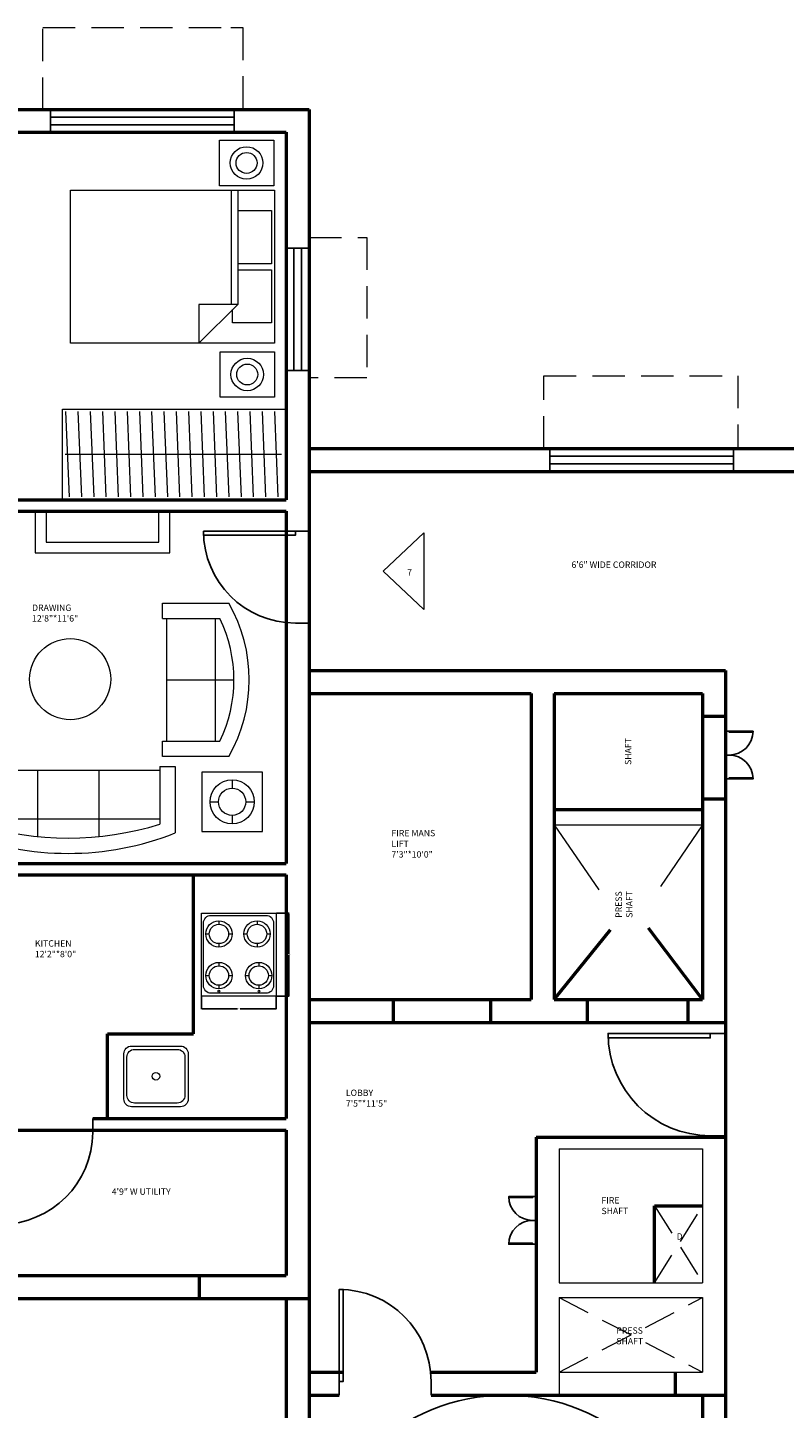
# Model space of a CAD drawing. Units: inches. Extents: x 4795 to 6024, y 2716 to 5025.
# Tile 14 of 19: x 5177 to 5473, y 4465 to 5006. Entities that reach past the tile are written whole.
import ezdxf

# ---------------------------------------------------------------- set-up
doc = ezdxf.new("R2010")
doc.units = ezdxf.units.IN
doc.linetypes.add('DASHED', pattern=[19.05, 12.7, -6.35])
for name, color, linetype, lineweight in [('A-ANNO-DIMS', 2, 'Continuous', 18), ('A-ANNO-TEXT', 7, 'Continuous', 18), ('A-AREA-IDEN', 3, 'Continuous', 18), ('A-DOOR', 4, 'Continuous', 25), ('A-FLOR-FIXT', 9, 'Continuous', 18), ('A-FLOR-STRS', 3, 'Continuous', 25), ('A-FURN', 8, 'Continuous', 18), ('A-GLAZ', 4, 'Continuous', 25), ('A-WALL', 7, 'Continuous', 50), ('A-WALL-OVHD', 8, 'DASHED', 18)]:
    doc.layers.add(name, color=color, linetype=linetype, lineweight=lineweight)
doc.styles.get("Standard").update_dxf_attribs({"font": 'arial.ttf'})
doc.dimstyles.get("Standard").update_dxf_attribs({"dimtxt": 0.18, "dimasz": 0.18, "dimexe": 0.18, "dimexo": 0.0625, "dimgap": 0.09, "dimtad": 0, "dimtih": 1, "dimtoh": 1, "dimdec": 4, "dimzin": 0, "dimdsep": 46, "dimtxsty": 'Standard', "dimcen": 0.09, "dimadec": 0, "dimazin": 0, "dimtfac": 1, "dimtdec": 4, "dimtofl": 0, "dimtmove": 0, "dimatfit": 3, "dimfxl": 1, "dimtolj": 1, "dimtzin": 0, "dimarcsym": 0})

# ---------------------------------------------------------------- blocks, each defined once
blk = doc.blocks.new('*U2')
for p, q in [((0, 0), (0, -6)), ((40, 0), (40, -6))]:
    blk.add_line(p, q)
blk.add_lwpolyline([(0, 0), (0, 40), (1.75, 40), (1.75, 0)], close=True)
blk.add_arc((0, 0), 40, 0, 90)
blk = doc.blocks.new('Bed - Queen')
for p, q in [((0, -80.00003), (0, 0)), ((0, 0), (59.99999, 0)), ((59.99999, 0), (59.99999, -80.00003)), ((7.99999, -1.2), (28.79998, -1.2)), ((7.99999, -14.4), (7.99999, -1.2)), ((28.79998, -1.2), (28.79998, -14.4)), ((31.19999, -1.2), (51.99999, -1.2)), ((31.19999, -14.4), (31.19999, -1.2)), ((51.99999, -1.2), (51.99999, -16.4)), ((0, -14.4), (44.8, -14.4)), ((59.99999, -29.6), (44.8, -14.4)), ((44.8, -14.4), (44.8, -29.6)), ((44.8, -16.8), (0, -16.8)), ((51.99999, -16.4), (46.79936, -16.4)), ((44.8, -29.6), (59.99999, -29.6)), ((59.99999, -80.00003), (0, -80.00003))]:
    blk.add_line(p, q)
blk = doc.blocks.new('Sofa - Roundback 7 ft.')
for p, q in [((-12.00002, -32.4421), (-12.00003, -6.5971)), ((11.99997, -32.4421), (11.99998, -6.5971)), ((-36.000027, -34), (-36.000027, -11.4696)), ((-35.999844, -13.3819), (35.9998, -13.3819)), ((35.99998, -34), (35.99998, -11.4696)), ((-36.000027, -32.4421), (35.99998, -32.4421))]:
    blk.add_line(p, q)
for points in [[(-36.000027, -34), (-42.000027, -34), (-42.000027, -8)], [(41.99998, -8), (41.99998, -34), (35.99998, -34)]]:
    blk.add_lwpolyline(points)
for centre, radius, start, end in [((0, -114.25), 114.25, 68.43141, 111.5686), ((-0.00001, -127.1968), 121.1968, 72.72033, 107.2797)]:
    blk.add_arc(centre, radius, start, end)
blk = doc.blocks.new('Sofa - Roundback Loveseat 5 ft.')
for p, q in [((0, -32.44198), (0, -5.99998)), ((-24, -33.99998), (-24, -11.46958)), ((-23.9998, -13.38178), (23.99986, -13.38178)), ((24.00004, -33.99998), (24.00004, -11.46958)), ((-24, -32.44198), (24.00004, -32.44198))]:
    blk.add_line(p, q)
for points in [[(-24, -33.99998), (-30, -33.99998), (-30, -7.99998)], [(30.00004, -7.99998), (30.00004, -33.99998), (24.00004, -33.99998)]]:
    blk.add_lwpolyline(points)
for centre, radius, start, end in [((0, -60.24998), 60.24998, 60.13715, 119.8628), ((0, -61.38438), 55.38444, 64.32083, 115.6792)]:
    blk.add_arc(centre, radius, start, end)
blk = doc.blocks.new('WIN-48')
for p, q in [((0, 0), (0, 48)), ((0, 48), (9, 48)), ((3, 0), (3, 48)), ((6, 48), (6, 0)), ((9, 48), (9, 0)), ((9, 0), (0, 0))]:
    blk.add_line(p, q)
blk = doc.blocks.new('WIN-72')
for p, q in [((0, 0), (0, 9)), ((0, 9), (72, 9)), ((0, 6), (72, 6)), ((72, 9), (72, 0)), ((72, 3), (0, 3)), ((72, 0), (0, 0))]:
    blk.add_line(p, q)
blk = doc.blocks.new('COOKTOP-4B')
for p, q in [((6.77, 29.57), (6.77, 28.22)), ((21.7, 29.57), (21.7, 28.22)), ((1.61, 24.41), (2.97, 24.41)), ((10.57, 24.41), (11.93, 24.41)), ((16.54, 24.41), (17.9, 24.41)), ((25.51, 24.41), (26.87, 24.41)), ((6.77, 20.61), (6.77, 19.25)), ((21.7, 20.61), (21.7, 19.25)), ((6.77, 13.27), (6.77, 11.91)), ((22.37, 13.27), (22.37, 11.91)), ((1.61, 8.11), (2.97, 8.11)), ((10.57, 8.11), (11.93, 8.11)), ((17.2, 8.11), (18.56, 8.11)), ((26.17, 8.11), (27.53, 8.11)), ((6.77, 4.3), (6.77, 2.94)), ((22.37, 4.3), (22.37, 2.94))]:
    blk.add_line(p, q)
blk.add_lwpolyline([(0, 32.52), (29.24, 32.52), (29.24, 0), (0, 0)], close=True)
blk.add_lwpolyline([(3.72, 31.71), (25.19, 31.71, -0.414214), (28.19, 28.71), (28.19, 4.17, -0.414214), (25.19, 1.17), (3.72, 1.17, -0.414214), (0.72, 4.17), (0.72, 28.71, -0.414214)], format="xyb", close=True)
for centre, radius in [((6.77, 24.41), 5.16), ((6.77, 24.41), 3.8), ((21.7, 24.41), 5.16), ((21.7, 24.41), 3.8), ((6.77, 8.11), 5.16), ((6.77, 8.11), 3.8), ((22.37, 8.11), 5.16), ((22.37, 8.11), 3.8), ((6.77, 2), 0.353), ((22.47, 2), 0.353)]:
    blk.add_circle(centre, radius)
blk = doc.blocks.new('LAMP-SIDE')
for p, q in [((11.88, 20.25), (11.88, 16.92)), ((3.23, 11.6), (6.56, 11.6)), ((17.2, 11.6), (20.54, 11.6)), ((11.88, 6.28), (11.88, 2.94))]:
    blk.add_line(p, q)
blk.add_lwpolyline([(23.76, 23.19), (0, 23.19), (0, 0), (23.76, 0)], close=True)
for radius in [8.66, 5.32]:
    blk.add_circle((11.88, 11.6), radius)
blk = doc.blocks.new('*D21')
at = {"layer": 'A-ANNO-DIMS', "color": 0, "lineweight": -2, "transparency": 16777216}
for p, q in [((5274.14, 4658.94), (5279.14, 4658.94)), ((5278.96, 4658.76), (5278.96, 4642.86)), ((5278.96, 4626.59), (5278.96, 4642.49)), ((5274.14, 4626.41), (5279.14, 4626.41))]:
    blk.add_line(p, q, dxfattribs=at)
at = {"layer": 'A-ANNO-DIMS', "color": 0, "lineweight": 100, "transparency": 16777216}
for points in [[(5278.93, 4658.76), (5278.99, 4658.76), (5278.96, 4658.94)], [(5278.93, 4626.59), (5278.99, 4626.59), (5278.96, 4626.41)]]:
    blk.add_solid(points, dxfattribs=at)
at = {"layer": 'DEFPOINTS', "color": 0, "lineweight": 100, "transparency": 16777216}
for p in [(5274.08, 4658.94), (5278.96, 4658.94), (5274.08, 4626.41)]:
    blk.add_point(p, dxfattribs=at)
at = {"layer": 'A-ANNO-DIMS', "color": 0, "transparency": 16777216, "insert": (5278.96, 4642.67), "char_height": 0.18, "attachment_point": 5}
blk.add_mtext('\\A1;COOKTOP 33 TYP.', dxfattribs=at)
blk = doc.blocks.new('*D22')
at = {"layer": 'A-ANNO-DIMS', "color": 0, "lineweight": -2, "transparency": 16777216}
for p, q in [((5244.83, 4626.35), (5244.83, 4621.35)), ((5245.01, 4621.53), (5258.93, 4621.53)), ((5273.9, 4621.53), (5259.99, 4621.53)), ((5274.08, 4626.35), (5274.08, 4621.35))]:
    blk.add_line(p, q, dxfattribs=at)
at = {"layer": 'A-ANNO-DIMS', "color": 0, "lineweight": 100, "transparency": 16777216}
for points in [[(5245.01, 4621.56), (5245.01, 4621.5), (5244.83, 4621.53)], [(5273.9, 4621.56), (5273.9, 4621.5), (5274.08, 4621.53)]]:
    blk.add_solid(points, dxfattribs=at)
at = {"layer": 'DEFPOINTS', "color": 0, "lineweight": 100, "transparency": 16777216}
for p in [(5244.83, 4626.41), (5274.08, 4626.41), (5274.08, 4621.53)]:
    blk.add_point(p, dxfattribs=at)
at = {"layer": 'A-ANNO-DIMS', "color": 0, "transparency": 16777216, "insert": (5259.46, 4621.53), "char_height": 0.18, "attachment_point": 5}
blk.add_mtext('\\A1;29 TYP.', dxfattribs=at)

msp = doc.modelspace()

# ---------------------------------------------------------------- linework, layer by layer
at = {"layer": 'A-FLOR-FIXT'}
for points in [[(5217.35, 4606.89), (5236.56, 4606.89, -0.414214), (5239.56, 4603.89), (5239.56, 4586.09, -0.414214), (5236.56, 4583.09), (5217.35, 4583.09, -0.414214), (5214.35, 4586.09), (5214.35, 4603.89, -0.414214)], [(5218.54, 4605.58), (5235.28, 4605.58, -0.414214), (5238.28, 4602.58), (5238.28, 4587.56, -0.414214), (5235.28, 4584.56), (5218.54, 4584.56, -0.414214), (5215.54, 4587.56), (5215.54, 4602.58, -0.414214)]]:
    msp.add_lwpolyline(points, format="xyb", close=True, dxfattribs=at)
msp.add_circle((5226.91, 4595.07), 1.48, dxfattribs=at)
at = {"layer": 'A-FLOR-STRS'}
msp.add_arc((5364.1, 4392.81), 77.28, 3.6633, 176.3367, dxfattribs=at)
at = {"layer": 'A-FURN'}
for p, q in [((5190.23, 4820.98), (5190.23, 4856.49)), ((5190.23, 4856.49), (5277.97, 4856.49)), ((5191.53, 4855.62), (5192.9, 4822.09)), ((5196.35, 4855.62), (5197.71, 4822.09)), ((5201.16, 4855.62), (5202.53, 4822.09)), ((5205.97, 4855.62), (5207.34, 4822.09)), ((5210.78, 4855.62), (5212.15, 4822.09)), ((5215.6, 4855.62), (5216.96, 4822.09)), ((5220.41, 4855.62), (5221.78, 4822.09)), ((5225.22, 4855.62), (5226.59, 4822.09)), ((5230.04, 4855.62), (5231.4, 4822.09)), ((5234.85, 4855.62), (5236.21, 4822.09)), ((5239.66, 4855.62), (5241.03, 4822.09)), ((5244.47, 4855.62), (5245.84, 4822.09)), ((5249.29, 4855.62), (5250.65, 4822.09)), ((5254.1, 4855.62), (5255.47, 4822.09)), ((5258.91, 4855.62), (5260.28, 4822.09)), ((5263.72, 4855.62), (5265.09, 4822.09)), ((5268.54, 4855.62), (5269.9, 4822.09)), ((5273.35, 4855.62), (5274.72, 4822.09)), ((5191.32, 4838.86), (5276.09, 4838.86)), ((5179.57, 4816.48), (5179.57, 4800.19)), ((5183.83, 4816.48), (5183.83, 4804.4)), ((5228.09, 4804.4), (5228.09, 4816.48)), ((5232.41, 4800.19), (5232.41, 4816.48)), ((5315.98, 4793.05), (5331.91, 4808.07)), ((5331.91, 4808.07), (5331.91, 4778.02)), ((5179.57, 4800.19), (5232.41, 4800.19)), ((5183.83, 4804.4), (5228.09, 4804.4)), ((5331.91, 4778.02), (5315.98, 4793.05)), ((5382.97, 4693.53), (5441.22, 4693.53)), ((5382.97, 4693.53), (5400.54, 4668.09)), ((5441.22, 4693.53), (5424.68, 4669.42)), ((5384.97, 4566.65), (5384.97, 4514.14)), ((5384.97, 4566.65), (5441.22, 4566.65)), ((5441.22, 4566.65), (5441.22, 4514.14)), ((5384.97, 4514.14), (5441.22, 4514.14)), ((5384.97, 4508.3), (5441.22, 4508.3)), ((5384.97, 4508.3), (5384.97, 4479.09)), ((5441.22, 4508.3), (5441.22, 4479.09)), ((5384.97, 4479.09), (5441.22, 4479.09)), ((5384.97, 4479.09), (5384.97, 4470.09))]:
    msp.add_line(p, q, dxfattribs=at)
for points in [[(5251.8, 4961.89), (5273.07, 4961.89), (5273.07, 4944.06), (5251.8, 4944.06)], [(5252.07, 4878.99), (5273.33, 4878.99), (5273.33, 4861.16), (5252.07, 4861.16)]]:
    msp.add_lwpolyline(points, close=True, dxfattribs=at)
for centre, radius in [((5262.44, 4952.98), 6.37), ((5262.44, 4952.98), 4.11), ((5262.7, 4870.07), 6.37), ((5262.7, 4870.07), 4.11), ((5193.31, 4750.68), 15.92)]:
    msp.add_circle(centre, radius, dxfattribs=at)
at = {"layer": 'A-WALL'}
for p, q in [((5133.97, 4973.98), (5286.97, 4973.98)), ((5286.97, 4973.98), (5286.97, 4507.98)), ((5133.97, 4964.98), (5277.97, 4964.98)), ((5277.97, 4964.98), (5277.97, 4820.98)), ((5286.97, 4841.09), (5528.22, 4841.09)), ((5286.97, 4832.09), (5528.22, 4832.09)), ((5129.47, 4820.98), (5277.97, 4820.98)), ((5129.47, 4816.48), (5277.97, 4816.48)), ((5277.97, 4816.48), (5277.97, 4678.48)), ((5286.97, 4754.09), (5450.22, 4754.09)), ((5450.22, 4754.09), (5450.22, 4616.09)), ((5286.97, 4745.09), (5373.97, 4745.09)), ((5373.97, 4745.09), (5373.97, 4625.09)), ((5382.97, 4745.09), (5382.97, 4625.09)), ((5382.97, 4745.09), (5441.22, 4745.09)), ((5441.22, 4745.09), (5441.22, 4625.09)), ((5441.22, 4736.21), (5450.22, 4736.21)), ((5441.22, 4703.73), (5450.22, 4703.73)), ((5382.97, 4699.56), (5441.22, 4699.56)), ((5128.97, 4678.48), (5277.97, 4678.48)), ((5128.97, 4673.98), (5277.97, 4673.98)), ((5241.6, 4611.62), (5241.6, 4673.98)), ((5277.97, 4673.98), (5277.97, 4578.48)), ((5382.97, 4625.09), (5405.07, 4652.47)), ((5441.22, 4625.09), (5419.93, 4653.06)), ((5286.97, 4625.09), (5373.97, 4625.09)), ((5319.94, 4625.09), (5319.94, 4616.09)), ((5358.12, 4625.09), (5358.12, 4616.09)), ((5382.97, 4625.09), (5441.22, 4625.09)), ((5395.95, 4625.09), (5395.95, 4616.09)), ((5435.43, 4625.09), (5435.43, 4616.09)), ((5286.97, 4616.09), (5450.22, 4616.09)), ((5450.22, 4616.09), (5450.22, 4571.15)), ((5207.97, 4578.48), (5207.97, 4611.62)), ((5207.97, 4611.62), (5241.6, 4611.62)), ((5202.12, 4578.48), (5277.97, 4578.48)), ((5133.47, 4573.98), (5277.97, 4573.98)), ((5277.97, 4573.98), (5277.97, 4516.98)), ((5375.97, 4571.15), (5375.97, 4479.09)), ((5375.97, 4571.15), (5450.22, 4571.15)), ((5450.22, 4571.15), (5450.22, 4470.09)), ((5422.37, 4514.14), (5422.37, 4544.27)), ((5422.37, 4544.27), (5441.22, 4544.27)), ((5133.47, 4516.98), (5277.97, 4516.98)), ((5243.82, 4516.98), (5243.82, 4507.98)), ((5161.01, 4507.98), (5286.97, 4507.98)), ((5277.97, 4507.98), (5277.97, 4368.81)), ((5286.97, 4507.98), (5286.97, 4507.98)), ((5286.97, 4507.98), (5286.97, 4223.31)), ((5286.97, 4479.09), (5300.36, 4479.09)), ((5334.6, 4479.09), (5375.97, 4479.09)), ((5430.4, 4479.09), (5430.4, 4470.09)), ((5286.97, 4470.09), (5298.78, 4470.09)), ((5334.78, 4470.09), (5450.22, 4470.09)), ((5441.22, 4470.09), (5441.22, 4240.93)), ((5450.22, 4470.09), (5450.22, 4231.93))]:
    msp.add_line(p, q, dxfattribs=at)
at = {"layer": 'A-WALL-OVHD'}
for p, q in [((5182.61, 4973.76), (5182.61, 5006.01)), ((5182.61, 5006.01), (5256.31, 5006.01)), ((5256.31, 5006.01), (5261, 5006.01)), ((5261, 5006.01), (5261, 4973.98)), ((5286.97, 4923.74), (5309.57, 4923.74)), ((5309.57, 4923.74), (5309.57, 4868.81)), ((5309.57, 4868.81), (5286.97, 4868.81)), ((5378.96, 4841.09), (5378.96, 4869.57)), ((5378.96, 4869.57), (5455.03, 4869.57)), ((5455.03, 4869.57), (5455.03, 4841.09)), ((5422.37, 4544.27), (5441.22, 4514.14)), ((5422.37, 4514.14), (5441.22, 4544.27)), ((5384.97, 4508.3), (5441.22, 4479.09)), ((5384.97, 4479.09), (5441.22, 4508.3))]:
    msp.add_line(p, q, dxfattribs=at)

# ---------------------------------------------------------------- block references
at = {"layer": 'A-DOOR'}
for p, xscale, yscale, zscale, rotation in [((5281.57, 4808.67), -0.9, 0.9, 0.9, 90), ((5451.62, 4730.29), 0.2337145210718518, 0.2337145210718518, 0.2337145210718518, 270), ((5451.62, 4711.6), -0.2337145210718518, 0.2337145210718518, 0.2337145210718518, 270), ((5444.21, 4611.83), -1.001833080642633, 1.001833080642633, 1.001833080642633, 90), ((5166.12, 4573.08), -0.9, 0.9, 0.9, 180), ((5374.57, 4547.9), -0.2337145210718518, 0.2337145210718518, 0.2337145210718518, 90), ((5374.57, 4529.2), 0.2337145210718518, 0.2337145210718518, 0.2337145210718518, 89.99999999999999)]:
    msp.add_blockref('*U2', p, dxfattribs=dict(at, xscale=xscale, yscale=yscale, zscale=zscale, rotation=rotation))
at = {"layer": 'A-DOOR', "xscale": 0.9, "yscale": 0.9, "zscale": 0.9}
msp.add_blockref('*U2', (5298.78, 4475.49), dxfattribs=at)
at = {"layer": 'A-FLOR-FIXT'}
msp.add_blockref('COOKTOP-4B', (5244.84, 4626.41), dxfattribs=at)
at = {"layer": 'A-FURN'}
for name, p, rotation in [('Bed - Queen', (5273.39, 4942.29), 270), ('Sofa - Roundback Loveseat 5 ft.', (5263.49, 4750.4), 270), ('Sofa - Roundback 7 ft.', (5192.5, 4682.4), 180)]:
    msp.add_blockref(name, p, dxfattribs=dict(at, rotation=rotation))
msp.add_blockref('LAMP-SIDE', (5244.9, 4691.01), dxfattribs=at)
at = {"layer": 'A-GLAZ', "rotation": 180}
for p in [(5257.63, 4973.98), (5453.31, 4841.09)]:
    msp.add_blockref('WIN-72', p, dxfattribs=at)
at = {"layer": 'A-GLAZ'}
msp.add_blockref('WIN-48', (5277.97, 4871.58), dxfattribs=at)

# ---------------------------------------------------------------- texts
at = {"layer": 'A-ANNO-TEXT', "char_height": 2.5, "attachment_point": 1}
for s, width, insert in [('7', 7.243, (5325.38, 4793.74)), ('D', 1.3867, (5431.02, 4533.53))]:
    msp.add_mtext_dynamic_manual_height_columns(s, width=width, gutter_width=12.5, heights=[0], dxfattribs=dict(at, insert=insert))
at = {"layer": 'A-AREA-IDEN', "char_height": 2.5, "attachment_point": 1}
for s, width, insert in [('6\'6" WIDE CORRIDOR', 114.2605, (5389.79, 4796.79)), ('DRAWING\\P12\'8"*11\'6"', 30.8983, (5178.36, 4779.92)), ('FIRE MANS\\PLIFT\\P7\'3"*10\'0"', 50.1224, (5319.24, 4691.6)), ('KITCHEN\\P12\'2"*8\'0"', 46.3011, (5179.47, 4648.37)), ('LOBBY\\P7\'5"*11\'5"', 56.2114, (5301.37, 4589.83)), ('4\'9" W UTILITY', 48.155, (5209.61, 4551.09)), ('FIRE\\PSHAFT', 26.113, (5401.55, 4547.69)), ('PRESS\\PSHAFT', 30.5555, (5407.38, 4496.67))]:
    msp.add_mtext_dynamic_manual_height_columns(s, width=width, gutter_width=12.5, heights=[0], dxfattribs=dict(at, insert=insert))
at = {"layer": 'A-AREA-IDEN', "char_height": 2.5, "attachment_point": 1, "rotation": 90}
for s, width, insert in [('SHAFT', 34.9976, (5410.74, 4717.07)), ('PRESS \\PSHAFT', 30.0186, (5407.05, 4657.14))]:
    msp.add_mtext_dynamic_manual_height_columns(s, width=width, gutter_width=12.5, heights=[0], dxfattribs=dict(at, insert=insert))

# ---------------------------------------------------------------- dimensions: what is measured, and where the dimension line sits
at = {"layer": 'A-ANNO-DIMS'}
dim = msp.add_linear_dim(base=(5278.96, 4658.94), p1=(5274.08, 4626.41), p2=(5274.08, 4658.94), angle=90, text='COOKTOP <> TYP.', dimstyle='Standard', override={"dimdec": 0, "dimlfac": 1, "dimrnd": 0, "dimzin": 0, "dimdsep": 46, "dimlunit": 2}, dxfattribs=at)
dim.commit()
dim.dimension.update_dxf_attribs({"geometry": '*D21', "text_midpoint": (5278.96, 4642.67)})
dim = msp.add_linear_dim(base=(5274.08, 4621.53), p1=(5244.83, 4626.41), p2=(5274.08, 4626.41), text='<> TYP.', dimstyle='Standard', override={"dimdec": 0, "dimlfac": 1, "dimrnd": 0, "dimzin": 0, "dimdsep": 46, "dimlunit": 2}, dxfattribs=at)
dim.commit()
dim.dimension.update_dxf_attribs({"geometry": '*D22', "text_midpoint": (5259.46, 4621.53)})

doc.saveas('drawing.dxf')
